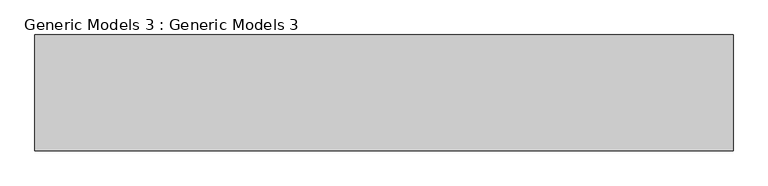
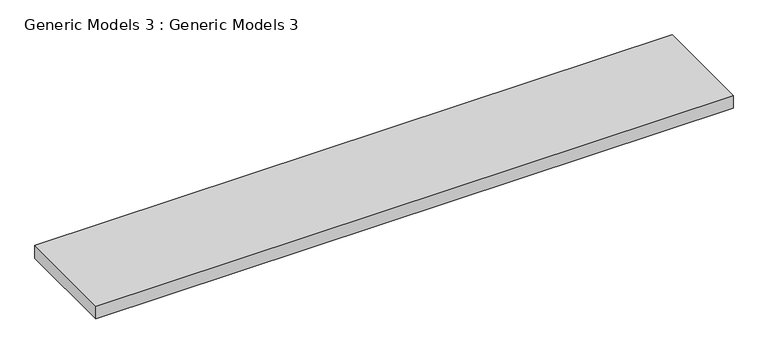
"""IFC4 building model written with IfcOpenShell, lengths in millimetres: proxy geometry, Generic Models 3 : Generic Models 3."""

from ifc_helpers import new_model, si_unit, frame, origin, place, context, project, spatial, polyline, outline, extrude, source, transform, mapped, element, save


def generic_models_3_generic_models_3_c7f04afc(model_context):
    return source(origin(), model_context, "Body", "SweptSolid", [
        extrude(outline(polyline([(10816.1582871, 14968.9102514), (-3765.0254981, 14968.9102514), (-3765.0254981, 17386.3), (10816.1582871, 17386.3), (10816.1582871, 14968.9102514)])), frame((0.0, 0.0, -76.2), z_axis=(0.0, 0.0, 1.0), x_axis=(1.0, 0.0, 0.0)), (0.0, 0.0, 1.0), 304.8),
    ])


if __name__ == "__main__":
    model = new_model("IFC4")
    model_context = context("Model", 3, world=origin())
    ifc_project = project(units=[si_unit("LENGTHUNIT", "METRE", prefix="MILLI")], contexts=[model_context])
    site = spatial("IfcSite", under=ifc_project)
    building = spatial("IfcBuilding", under=site)
    placement = place(None, origin())
    generic_models_3_generic_models_3_shape = generic_models_3_generic_models_3_c7f04afc(model_context)
    element("IfcBuildingElementProxy", 1, Name="Generic Models 3 : Generic Models 3", ObjectType="Generic Models 3 : Generic Models 3", at=placement, inside=building, context=model_context, shape_type="MappedRepresentation", body=[
        mapped(generic_models_3_generic_models_3_shape, transform((0.0, 0.0, 0.0), x_axis=(1.0, 0.0, 0.0), y_axis=(0.0, 1.0, 0.0), z_axis=(0.0, 0.0, 1.0))),
    ])
    save(model, "model.ifc")
